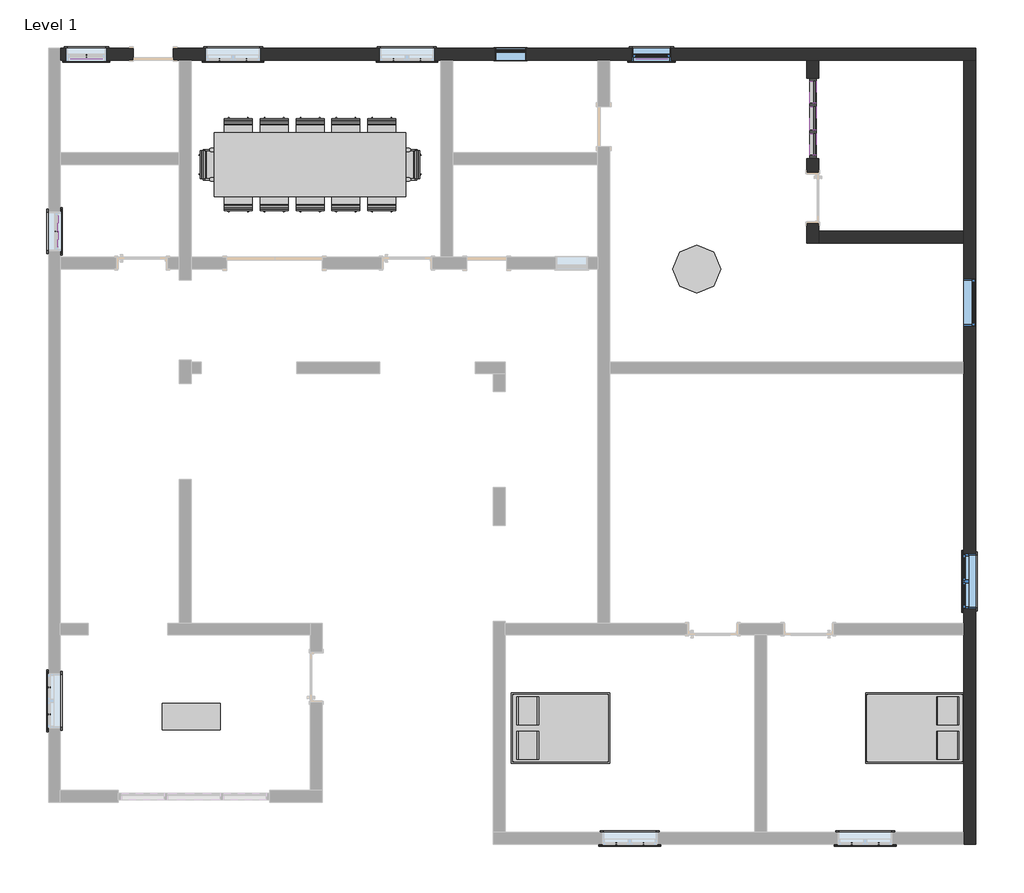
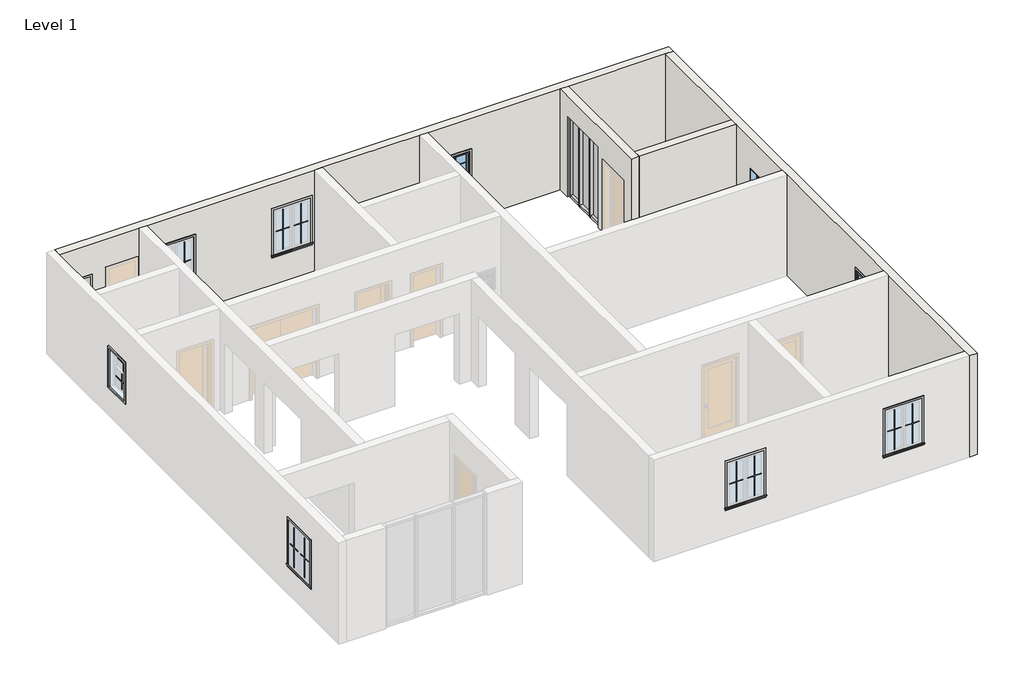
# One storey, part 2 of 2: 36 proxies, 17 furniture elements, 10 members, 4 walls, 4 windows, 3 plates.
"""IFC4 building model written with IfcOpenShell, lengths in millimetres."""

from ifc_helpers import new_model, si_unit, origin, origin_with_axes, place, context, project, spatial, polyline, outline, extrude, faceted_brep, transform, mapped, element, save
from components import muntin_pattern_2x2_muntin_pattern_2x2_88bf7f41, muntin_pattern_2x2_muntin_pattern_2x2_3dfd0a47, muntin_pattern_2x2_muntin_pattern_2x2_b8ba09c9, trim_window_exterior_flat_with_sill_4930676f, trim_window_exterior_flat_with_sill_6cd3ad68, trim_window_interior_flat_picture_frame_dd064338, trim_window_interior_flat_picture_frame_840a62db, furniture_b58f7881, chair_task_chair_task_b7f3823b, chair_task_arms_chair_task_arms_fa5a08ef, furniture_74675f9f, furniture_00fa8475, furniture_52f35bf4, member_05170f4c, member_f0fea5a5, member_24b1c93a, member_ee409385, system_panel_glazed_1f7552f7, system_panel_glazed_383feac9, window_c1f32544, window_c95ebb39, window_d400040f, window_f2d8fef0

model = new_model("IFC4")

# Units and contexts
model_context = context("Model", 3, world=origin())
ifc_project = project(units=[si_unit("LENGTHUNIT", "METRE", prefix="MILLI")], contexts=[model_context])

# Site, building, storey
site = spatial("IfcSite", under=ifc_project)
building = spatial("IfcBuilding", under=site)
storey = spatial("IfcBuildingStorey", under=building, Name="Level 1", Elevation=0.0)

# Proxies
placement = place(None, origin())
muntin_pattern_2x2_muntin_pattern_2x2_shape = muntin_pattern_2x2_muntin_pattern_2x2_88bf7f41(model_context)
element("IfcBuildingElementProxy", 1, Name="Muntin Pattern_2x2 : Muntin Pattern_2x2", ObjectType="Muntin Pattern_2x2 : Muntin Pattern_2x2", at=placement, inside=storey, context=model_context, shape_type="MappedRepresentation", body=[
    mapped(muntin_pattern_2x2_muntin_pattern_2x2_shape, transform((-3681.6839291, -4572.3847851, 984.25), x_axis=(-1.0, 0.0, 0.0), y_axis=(0.0, -1.0, 0.0), z_axis=(0.0, 0.0, 1.0))),
])
element("IfcBuildingElementProxy", 2, Name="Muntin Pattern_2x2 : Muntin Pattern_2x2", ObjectType="Muntin Pattern_2x2 : Muntin Pattern_2x2", at=placement, inside=storey, context=model_context, shape_type="MappedRepresentation", body=[
    mapped(muntin_pattern_2x2_muntin_pattern_2x2_shape, transform((818.2832584, -4572.3847851, 984.25), x_axis=(-1.0, 0.0, 0.0), y_axis=(0.0, -1.0, 0.0), z_axis=(0.0, 0.0, 1.0))),
])
element("IfcBuildingElementProxy", 3, Name="Muntin Pattern_2x2 : Muntin Pattern_2x2", ObjectType="Muntin Pattern_2x2 : Muntin Pattern_2x2", at=placement, inside=storey, context=model_context, shape_type="MappedRepresentation", body=[
    mapped(muntin_pattern_2x2_muntin_pattern_2x2_shape, transform((2454.7477116, 188.0316212, 984.25), x_axis=(0.0, 1.0, 0.0), y_axis=(-1.0, 0.0, 0.0), z_axis=(0.0, 0.0, 1.0))),
])
element("IfcBuildingElementProxy", 4, Name="Muntin Pattern_2x2 : Muntin Pattern_2x2", ObjectType="Muntin Pattern_2x2 : Muntin Pattern_2x2", at=placement, inside=storey, context=model_context, shape_type="MappedRepresentation", body=[
    mapped(muntin_pattern_2x2_muntin_pattern_2x2_shape, transform((-15045.2569759, -2097.9683788, 984.25), x_axis=(0.0, 1.0, 0.0), y_axis=(-1.0, 0.0, 0.0), z_axis=(0.0, 0.0, 1.0))),
])
element("IfcBuildingElementProxy", 5, Name="Muntin Pattern_2x2 : Muntin Pattern_2x2", ObjectType="Muntin Pattern_2x2 : Muntin Pattern_2x2", at=placement, inside=storey, context=model_context, shape_type="MappedRepresentation", body=[
    mapped(muntin_pattern_2x2_muntin_pattern_2x2_shape, transform((-11267.3046322, 10427.7042774, 984.25), x_axis=(-1.0, 0.0, 0.0), y_axis=(0.0, -1.0, 0.0), z_axis=(0.0, 0.0, 1.0))),
])
element("IfcBuildingElementProxy", 6, Name="Muntin Pattern_2x2 : Muntin Pattern_2x2", ObjectType="Muntin Pattern_2x2 : Muntin Pattern_2x2", at=placement, inside=storey, context=model_context, shape_type="MappedRepresentation", body=[
    mapped(muntin_pattern_2x2_muntin_pattern_2x2_shape, transform((-7943.6749447, 10427.7042774, 984.25), x_axis=(-1.0, 0.0, 0.0), y_axis=(0.0, -1.0, 0.0), z_axis=(0.0, 0.0, 1.0))),
])
muntin_pattern_2x2_muntin_pattern_2x2_2_shape = muntin_pattern_2x2_muntin_pattern_2x2_3dfd0a47(model_context)
element("IfcBuildingElementProxy", 7, Name="Muntin Pattern_2x2 : Muntin Pattern_2x2", ObjectType="Muntin Pattern_2x2 : Muntin Pattern_2x2", at=placement, inside=storey, context=model_context, shape_type="MappedRepresentation", body=[
    mapped(muntin_pattern_2x2_muntin_pattern_2x2_2_shape, transform((-4199.2089291, -4572.3847851, 984.25), x_axis=(1.0, 0.0, 0.0), y_axis=(0.0, 1.0, 0.0), z_axis=(0.0, 0.0, 1.0))),
])
element("IfcBuildingElementProxy", 8, Name="Muntin Pattern_2x2 : Muntin Pattern_2x2", ObjectType="Muntin Pattern_2x2 : Muntin Pattern_2x2", at=placement, inside=storey, context=model_context, shape_type="MappedRepresentation", body=[
    mapped(muntin_pattern_2x2_muntin_pattern_2x2_2_shape, transform((300.7582584, -4572.3847851, 984.25), x_axis=(1.0, 0.0, 0.0), y_axis=(0.0, 1.0, 0.0), z_axis=(0.0, 0.0, 1.0))),
])
element("IfcBuildingElementProxy", 9, Name="Muntin Pattern_2x2 : Muntin Pattern_2x2", ObjectType="Muntin Pattern_2x2 : Muntin Pattern_2x2", at=placement, inside=storey, context=model_context, shape_type="MappedRepresentation", body=[
    mapped(muntin_pattern_2x2_muntin_pattern_2x2_2_shape, transform((2454.7477116, 705.5566212, 984.25), x_axis=(0.0, -1.0, 0.0), y_axis=(1.0, 0.0, 0.0), z_axis=(0.0, 0.0, 1.0))),
])
element("IfcBuildingElementProxy", 10, Name="Muntin Pattern_2x2 : Muntin Pattern_2x2", ObjectType="Muntin Pattern_2x2 : Muntin Pattern_2x2", at=placement, inside=storey, context=model_context, shape_type="MappedRepresentation", body=[
    mapped(muntin_pattern_2x2_muntin_pattern_2x2_2_shape, transform((-15045.2569759, -1580.4433788, 984.25), x_axis=(0.0, -1.0, 0.0), y_axis=(1.0, 0.0, 0.0), z_axis=(0.0, 0.0, 1.0))),
])
element("IfcBuildingElementProxy", 11, Name="Muntin Pattern_2x2 : Muntin Pattern_2x2", ObjectType="Muntin Pattern_2x2 : Muntin Pattern_2x2", at=placement, inside=storey, context=model_context, shape_type="MappedRepresentation", body=[
    mapped(muntin_pattern_2x2_muntin_pattern_2x2_2_shape, transform((-11784.8296322, 10427.7042774, 984.25), x_axis=(1.0, 0.0, 0.0), y_axis=(0.0, 1.0, 0.0), z_axis=(0.0, 0.0, 1.0))),
])
element("IfcBuildingElementProxy", 12, Name="Muntin Pattern_2x2 : Muntin Pattern_2x2", ObjectType="Muntin Pattern_2x2 : Muntin Pattern_2x2", at=placement, inside=storey, context=model_context, shape_type="MappedRepresentation", body=[
    mapped(muntin_pattern_2x2_muntin_pattern_2x2_2_shape, transform((-8461.1999447, 10427.7042774, 984.25), x_axis=(1.0, 0.0, 0.0), y_axis=(0.0, 1.0, 0.0), z_axis=(0.0, 0.0, 1.0))),
])
muntin_pattern_2x2_muntin_pattern_2x2_3_shape = muntin_pattern_2x2_muntin_pattern_2x2_b8ba09c9(model_context)
element("IfcBuildingElementProxy", 13, Name="Muntin Pattern_2x2 : Muntin Pattern_2x2", ObjectType="Muntin Pattern_2x2 : Muntin Pattern_2x2", at=placement, inside=storey, context=model_context, shape_type="MappedRepresentation", body=[
    mapped(muntin_pattern_2x2_muntin_pattern_2x2_3_shape, transform((-14861.1069759, 7141.9761524, 1520.825), x_axis=(0.0, -1.0, 0.0), y_axis=(1.0, 0.0, 0.0), z_axis=(0.0, 0.0, 1.0))),
])
element("IfcBuildingElementProxy", 14, Name="Muntin Pattern_2x2 : Muntin Pattern_2x2", ObjectType="Muntin Pattern_2x2 : Muntin Pattern_2x2", at=placement, inside=storey, context=model_context, shape_type="MappedRepresentation", body=[
    mapped(muntin_pattern_2x2_muntin_pattern_2x2_3_shape, transform((-14905.5569759, 7141.9761524, 990.6), x_axis=(0.0, -1.0, 0.0), y_axis=(1.0, 0.0, 0.0), z_axis=(0.0, 0.0, 1.0))),
])
element("IfcBuildingElementProxy", 15, Name="Muntin Pattern_2x2 : Muntin Pattern_2x2", ObjectType="Muntin Pattern_2x2 : Muntin Pattern_2x2", at=placement, inside=storey, context=model_context, shape_type="MappedRepresentation", body=[
    mapped(muntin_pattern_2x2_muntin_pattern_2x2_3_shape, transform((-14330.8819759, 10453.1042774, 1520.825), x_axis=(-1.0, 0.0, 0.0), y_axis=(0.0, -1.0, 0.0), z_axis=(0.0, 0.0, 1.0))),
])
element("IfcBuildingElementProxy", 16, Name="Muntin Pattern_2x2 : Muntin Pattern_2x2", ObjectType="Muntin Pattern_2x2 : Muntin Pattern_2x2", at=placement, inside=storey, context=model_context, shape_type="MappedRepresentation", body=[
    mapped(muntin_pattern_2x2_muntin_pattern_2x2_3_shape, transform((-14330.8819759, 10497.5542774, 990.6), x_axis=(-1.0, 0.0, 0.0), y_axis=(0.0, -1.0, 0.0), z_axis=(0.0, 0.0, 1.0))),
])
element("IfcBuildingElementProxy", 17, Name="Muntin Pattern_2x2 : Muntin Pattern_2x2", ObjectType="Muntin Pattern_2x2 : Muntin Pattern_2x2", at=placement, inside=storey, context=model_context, shape_type="MappedRepresentation", body=[
    mapped(muntin_pattern_2x2_muntin_pattern_2x2_3_shape, transform((-3526.0593197, 10453.1042774, 1520.825), x_axis=(-1.0, 0.0, 0.0), y_axis=(0.0, -1.0, 0.0), z_axis=(0.0, 0.0, 1.0))),
])
element("IfcBuildingElementProxy", 18, Name="Muntin Pattern_2x2 : Muntin Pattern_2x2", ObjectType="Muntin Pattern_2x2 : Muntin Pattern_2x2", at=placement, inside=storey, context=model_context, shape_type="MappedRepresentation", body=[
    mapped(muntin_pattern_2x2_muntin_pattern_2x2_3_shape, transform((-3526.0593197, 10497.5542774, 990.6), x_axis=(-1.0, 0.0, 0.0), y_axis=(0.0, -1.0, 0.0), z_axis=(0.0, 0.0, 1.0))),
])
trim_window_exterior_flat_with_sill_shape = trim_window_exterior_flat_with_sill_4930676f(model_context)
element("IfcBuildingElementProxy", 19, Name="Trim-Window-Exterior-Flat : with Sill", ObjectType="Trim-Window-Exterior-Flat : with Sill", at=placement, inside=storey, context=model_context, shape_type="MappedRepresentation", body=[
    mapped(trim_window_exterior_flat_with_sill_shape, transform((-3940.4464291, -4581.9097851, 2260.6), x_axis=(1.0, 0.0, 0.0), y_axis=(0.0, 0.0, 1.0), z_axis=(0.0, -1.0, 0.0))),
])
element("IfcBuildingElementProxy", 20, Name="Trim-Window-Exterior-Flat : with Sill", ObjectType="Trim-Window-Exterior-Flat : with Sill", at=placement, inside=storey, context=model_context, shape_type="MappedRepresentation", body=[
    mapped(trim_window_exterior_flat_with_sill_shape, transform((559.5207584, -4581.9097851, 2260.6), x_axis=(1.0, 0.0, 0.0), y_axis=(0.0, 0.0, 1.0), z_axis=(0.0, -1.0, 0.0))),
])
element("IfcBuildingElementProxy", 21, Name="Trim-Window-Exterior-Flat : with Sill", ObjectType="Trim-Window-Exterior-Flat : with Sill", at=placement, inside=storey, context=model_context, shape_type="MappedRepresentation", body=[
    mapped(trim_window_exterior_flat_with_sill_shape, transform((2445.2227116, 446.7941212, 2260.6), x_axis=(0.0, -1.0, 0.0), y_axis=(0.0, 0.0, 1.0), z_axis=(-1.0, 0.0, 0.0))),
])
element("IfcBuildingElementProxy", 22, Name="Trim-Window-Exterior-Flat : with Sill", ObjectType="Trim-Window-Exterior-Flat : with Sill", at=placement, inside=storey, context=model_context, shape_type="MappedRepresentation", body=[
    mapped(trim_window_exterior_flat_with_sill_shape, transform((-15054.7819759, -1839.2058788, 2260.6), x_axis=(0.0, -1.0, 0.0), y_axis=(0.0, 0.0, 1.0), z_axis=(-1.0, 0.0, 0.0))),
])
element("IfcBuildingElementProxy", 23, Name="Trim-Window-Exterior-Flat : with Sill", ObjectType="Trim-Window-Exterior-Flat : with Sill", at=placement, inside=storey, context=model_context, shape_type="MappedRepresentation", body=[
    mapped(trim_window_exterior_flat_with_sill_shape, transform((-11526.0671322, 10418.1792774, 2260.6), x_axis=(1.0, 0.0, 0.0), y_axis=(0.0, 0.0, 1.0), z_axis=(0.0, -1.0, 0.0))),
])
element("IfcBuildingElementProxy", 24, Name="Trim-Window-Exterior-Flat : with Sill", ObjectType="Trim-Window-Exterior-Flat : with Sill", at=placement, inside=storey, context=model_context, shape_type="MappedRepresentation", body=[
    mapped(trim_window_exterior_flat_with_sill_shape, transform((-8202.4374447, 10418.1792774, 2260.6), x_axis=(1.0, 0.0, 0.0), y_axis=(0.0, 0.0, 1.0), z_axis=(0.0, -1.0, 0.0))),
])
trim_window_exterior_flat_with_sill_2_shape = trim_window_exterior_flat_with_sill_6cd3ad68(model_context)
element("IfcBuildingElementProxy", 25, Name="Trim-Window-Exterior-Flat : with Sill", ObjectType="Trim-Window-Exterior-Flat : with Sill", at=placement, inside=storey, context=model_context, shape_type="MappedRepresentation", body=[
    mapped(trim_window_exterior_flat_with_sill_2_shape, transform((-14826.1819759, 7141.9761524, 2082.8), x_axis=(0.0, 1.0, 0.0), y_axis=(0.0, 0.0, 1.0), z_axis=(1.0, 0.0, 0.0))),
])
element("IfcBuildingElementProxy", 26, Name="Trim-Window-Exterior-Flat : with Sill", ObjectType="Trim-Window-Exterior-Flat : with Sill", at=placement, inside=storey, context=model_context, shape_type="MappedRepresentation", body=[
    mapped(trim_window_exterior_flat_with_sill_2_shape, transform((-14330.8819759, 10418.1792774, 2082.8), x_axis=(1.0, 0.0, 0.0), y_axis=(0.0, 0.0, 1.0), z_axis=(0.0, -1.0, 0.0))),
])
element("IfcBuildingElementProxy", 27, Name="Trim-Window-Exterior-Flat : with Sill", ObjectType="Trim-Window-Exterior-Flat : with Sill", at=placement, inside=storey, context=model_context, shape_type="MappedRepresentation", body=[
    mapped(trim_window_exterior_flat_with_sill_2_shape, transform((-3526.0593197, 10418.1792774, 2082.8), x_axis=(1.0, 0.0, 0.0), y_axis=(0.0, 0.0, 1.0), z_axis=(0.0, -1.0, 0.0))),
])
trim_window_interior_flat_picture_frame_shape = trim_window_interior_flat_picture_frame_dd064338(model_context)
element("IfcBuildingElementProxy", 28, Name="Trim-Window-Interior-Flat : Picture Frame", ObjectType="Trim-Window-Interior-Flat : Picture Frame", at=placement, inside=storey, context=model_context, shape_type="MappedRepresentation", body=[
    mapped(trim_window_interior_flat_picture_frame_shape, transform((-3940.4464291, -4353.3097851, 2260.6), x_axis=(-1.0, 0.0, 0.0), y_axis=(0.0, 0.0, 1.0), z_axis=(0.0, 1.0, 0.0))),
])
element("IfcBuildingElementProxy", 29, Name="Trim-Window-Interior-Flat : Picture Frame", ObjectType="Trim-Window-Interior-Flat : Picture Frame", at=placement, inside=storey, context=model_context, shape_type="MappedRepresentation", body=[
    mapped(trim_window_interior_flat_picture_frame_shape, transform((559.5207584, -4353.3097851, 2260.6), x_axis=(-1.0, 0.0, 0.0), y_axis=(0.0, 0.0, 1.0), z_axis=(0.0, 1.0, 0.0))),
])
element("IfcBuildingElementProxy", 30, Name="Trim-Window-Interior-Flat : Picture Frame", ObjectType="Trim-Window-Interior-Flat : Picture Frame", at=placement, inside=storey, context=model_context, shape_type="MappedRepresentation", body=[
    mapped(trim_window_interior_flat_picture_frame_shape, transform((2673.8227116, 446.7941212, 2260.6), x_axis=(0.0, 1.0, 0.0), y_axis=(0.0, 0.0, 1.0), z_axis=(1.0, 0.0, 0.0))),
])
element("IfcBuildingElementProxy", 31, Name="Trim-Window-Interior-Flat : Picture Frame", ObjectType="Trim-Window-Interior-Flat : Picture Frame", at=placement, inside=storey, context=model_context, shape_type="MappedRepresentation", body=[
    mapped(trim_window_interior_flat_picture_frame_shape, transform((-14826.1819759, -1839.2058788, 2260.6), x_axis=(0.0, 1.0, 0.0), y_axis=(0.0, 0.0, 1.0), z_axis=(1.0, 0.0, 0.0))),
])
element("IfcBuildingElementProxy", 32, Name="Trim-Window-Interior-Flat : Picture Frame", ObjectType="Trim-Window-Interior-Flat : Picture Frame", at=placement, inside=storey, context=model_context, shape_type="MappedRepresentation", body=[
    mapped(trim_window_interior_flat_picture_frame_shape, transform((-11526.0671322, 10646.7792774, 2260.6), x_axis=(-1.0, 0.0, 0.0), y_axis=(0.0, 0.0, 1.0), z_axis=(0.0, 1.0, 0.0))),
])
element("IfcBuildingElementProxy", 33, Name="Trim-Window-Interior-Flat : Picture Frame", ObjectType="Trim-Window-Interior-Flat : Picture Frame", at=placement, inside=storey, context=model_context, shape_type="MappedRepresentation", body=[
    mapped(trim_window_interior_flat_picture_frame_shape, transform((-8202.4374447, 10646.7792774, 2260.6), x_axis=(-1.0, 0.0, 0.0), y_axis=(0.0, 0.0, 1.0), z_axis=(0.0, 1.0, 0.0))),
])
trim_window_interior_flat_picture_frame_2_shape = trim_window_interior_flat_picture_frame_840a62db(model_context)
element("IfcBuildingElementProxy", 34, Name="Trim-Window-Interior-Flat : Picture Frame", ObjectType="Trim-Window-Interior-Flat : Picture Frame", at=placement, inside=storey, context=model_context, shape_type="MappedRepresentation", body=[
    mapped(trim_window_interior_flat_picture_frame_2_shape, transform((-15054.7819759, 7141.9761524, 2082.8), x_axis=(0.0, -1.0, 0.0), y_axis=(0.0, 0.0, 1.0), z_axis=(-1.0, 0.0, 0.0))),
])
element("IfcBuildingElementProxy", 35, Name="Trim-Window-Interior-Flat : Picture Frame", ObjectType="Trim-Window-Interior-Flat : Picture Frame", at=placement, inside=storey, context=model_context, shape_type="MappedRepresentation", body=[
    mapped(trim_window_interior_flat_picture_frame_2_shape, transform((-14330.8819759, 10646.7792774, 2082.8), x_axis=(-1.0, 0.0, 0.0), y_axis=(0.0, 0.0, 1.0), z_axis=(0.0, 1.0, 0.0))),
])
element("IfcBuildingElementProxy", 36, Name="Trim-Window-Interior-Flat : Picture Frame", ObjectType="Trim-Window-Interior-Flat : Picture Frame", at=placement, inside=storey, context=model_context, shape_type="MappedRepresentation", body=[
    mapped(trim_window_interior_flat_picture_frame_2_shape, transform((-3526.0593197, 10646.7792774, 2082.8), x_axis=(-1.0, 0.0, 0.0), y_axis=(0.0, 0.0, 1.0), z_axis=(0.0, 1.0, 0.0))),
])

# Furniture
furniture_shape = furniture_b58f7881(model_context)
element("IfcFurniture", 37, ObjectType="Bed-Box : Double 53\" x 74\"", at=placement, inside=storey, context=model_context, shape_type="MappedRepresentation", body=[
    mapped(furniture_shape, transform((-5500.3888279, -2699.0583378, 0.0), x_axis=(0.0, 1.0, 0.0), y_axis=(-1.0, 0.0, 0.0), z_axis=(0.0, 0.0, 1.0))),
])
element("IfcFurniture", 38, ObjectType="Bed-Box : Double 53\" x 74\"", at=placement, inside=storey, context=model_context, shape_type="MappedRepresentation", body=[
    mapped(furniture_shape, transform((1739.8522198, -2020.7534198, 0.0), x_axis=(0.0, -1.0, 0.0), y_axis=(1.0, 0.0, 0.0), z_axis=(0.0, 0.0, 1.0))),
])
chair_task_chair_task_shape = chair_task_chair_task_b7f3823b(model_context)
element("IfcFurniture", 39, ObjectType="Chair-Task : Chair-Task", at=placement, inside=storey, context=model_context, shape_type="MappedRepresentation", body=[
    mapped(chair_task_chair_task_shape, transform((-9227.9614688, 9046.5743978, 0.0), x_axis=(-1.0, 0.0, 0.0), y_axis=(0.0, -1.0, 0.0), z_axis=(0.0, 0.0, 1.0))),
])
element("IfcFurniture", 40, ObjectType="Chair-Task : Chair-Task", at=placement, inside=storey, context=model_context, shape_type="MappedRepresentation", body=[
    mapped(chair_task_chair_task_shape, transform((-9509.9431081, 7789.4825945, 0.0), x_axis=(1.0, 0.0, 0.0), y_axis=(0.0, 1.0, 0.0), z_axis=(0.0, 0.0, 1.0))),
])
element("IfcFurniture", 41, ObjectType="Chair-Task : Chair-Task", at=placement, inside=storey, context=model_context, shape_type="MappedRepresentation", body=[
    mapped(chair_task_chair_task_shape, transform((-9913.7614688, 9046.5743978, 0.0), x_axis=(-1.0, 0.0, 0.0), y_axis=(0.0, -1.0, 0.0), z_axis=(0.0, 0.0, 1.0))),
])
element("IfcFurniture", 42, ObjectType="Chair-Task : Chair-Task", at=placement, inside=storey, context=model_context, shape_type="MappedRepresentation", body=[
    mapped(chair_task_chair_task_shape, transform((-10195.7431081, 7789.4825945, 0.0), x_axis=(1.0, 0.0, 0.0), y_axis=(0.0, 1.0, 0.0), z_axis=(0.0, 0.0, 1.0))),
])
element("IfcFurniture", 43, ObjectType="Chair-Task : Chair-Task", at=placement, inside=storey, context=model_context, shape_type="MappedRepresentation", body=[
    mapped(chair_task_chair_task_shape, transform((-10599.5614688, 9046.5743978, 0.0), x_axis=(-1.0, 0.0, 0.0), y_axis=(0.0, -1.0, 0.0), z_axis=(0.0, 0.0, 1.0))),
])
element("IfcFurniture", 44, ObjectType="Chair-Task : Chair-Task", at=placement, inside=storey, context=model_context, shape_type="MappedRepresentation", body=[
    mapped(chair_task_chair_task_shape, transform((-8542.1614688, 9046.5743978, 0.0), x_axis=(-1.0, 0.0, 0.0), y_axis=(0.0, -1.0, 0.0), z_axis=(0.0, 0.0, 1.0))),
])
element("IfcFurniture", 45, ObjectType="Chair-Task : Chair-Task", at=placement, inside=storey, context=model_context, shape_type="MappedRepresentation", body=[
    mapped(chair_task_chair_task_shape, transform((-10881.5431081, 7789.4825945, 0.0), x_axis=(1.0, 0.0, 0.0), y_axis=(0.0, 1.0, 0.0), z_axis=(0.0, 0.0, 1.0))),
])
element("IfcFurniture", 46, ObjectType="Chair-Task : Chair-Task", at=placement, inside=storey, context=model_context, shape_type="MappedRepresentation", body=[
    mapped(chair_task_chair_task_shape, transform((-8824.1431081, 7789.4825945, 0.0), x_axis=(1.0, 0.0, 0.0), y_axis=(0.0, 1.0, 0.0), z_axis=(0.0, 0.0, 1.0))),
])
element("IfcFurniture", 47, ObjectType="Chair-Task : Chair-Task", at=placement, inside=storey, context=model_context, shape_type="MappedRepresentation", body=[
    mapped(chair_task_chair_task_shape, transform((-11285.3614688, 9046.5743978, 0.0), x_axis=(-1.0, 0.0, 0.0), y_axis=(0.0, -1.0, 0.0), z_axis=(0.0, 0.0, 1.0))),
])
element("IfcFurniture", 48, ObjectType="Chair-Task : Chair-Task", at=placement, inside=storey, context=model_context, shape_type="MappedRepresentation", body=[
    mapped(chair_task_chair_task_shape, transform((-11567.3431081, 7789.4825945, 0.0), x_axis=(1.0, 0.0, 0.0), y_axis=(0.0, 1.0, 0.0), z_axis=(0.0, 0.0, 1.0))),
])
chair_task_arms_chair_task_arms_shape = chair_task_arms_chair_task_arms_fa5a08ef(model_context)
element("IfcFurniture", 49, ObjectType="Chair-Task Arms : Chair-Task Arms", at=placement, inside=storey, context=model_context, shape_type="MappedRepresentation", body=[
    mapped(chair_task_arms_chair_task_arms_shape, transform((-11902.4981901, 8559.0193159, 0.0), x_axis=(0.0, -1.0, 0.0), y_axis=(1.0, 0.0, 0.0), z_axis=(0.0, 0.0, 1.0))),
])
element("IfcFurniture", 50, ObjectType="Chair-Task Arms : Chair-Task Arms", at=placement, inside=storey, context=model_context, shape_type="MappedRepresentation", body=[
    mapped(chair_task_arms_chair_task_arms_shape, transform((-8207.0063868, 8277.0376765, 0.0), x_axis=(0.0, 1.0, 0.0), y_axis=(-1.0, 0.0, 0.0), z_axis=(0.0, 0.0, 1.0))),
])
furniture_2_shape = furniture_74675f9f(model_context)
element("IfcFurniture", 51, ObjectType="Table-Coffee Mission : 44\" x 20\"", at=placement, inside=storey, context=model_context, shape_type="MappedRepresentation", body=[
    mapped(furniture_2_shape, transform((-12326.1671322, -2144.0058788, 0.0), x_axis=(1.0, 0.0, 0.0), y_axis=(0.0, 1.0, 0.0), z_axis=(0.0, 0.0, 1.0))),
])
furniture_3_shape = furniture_00fa8475(model_context)
element("IfcFurniture", 52, ObjectType="Table-Conference2 w Chairs : 48\" x 144\"", at=placement, inside=storey, context=model_context, shape_type="MappedRepresentation", body=[
    mapped(furniture_3_shape, transform((-10054.7522884, 8418.0284962, 0.0), x_axis=(1.0, 0.0, 0.0), y_axis=(0.0, 1.0, 0.0), z_axis=(0.0, 0.0, 1.0))),
])
furniture_4_shape = furniture_52f35bf4(model_context)
element("IfcFurniture", 53, ObjectType="Table-Dining Round w Chairs : 36\" Diameter", at=placement, inside=storey, context=model_context, shape_type="MappedRepresentation", body=[
    mapped(furniture_4_shape, transform((-2763.3631619, 6602.954841, 0.0), x_axis=(1.0, 0.0, 0.0), y_axis=(0.0, 1.0, 0.0), z_axis=(0.0, 0.0, 1.0))),
])

# Members
member_shape = member_05170f4c(model_context)
element("IfcMember", 54, ObjectType="Rectangular Mullion : 2.5\" x 5\" rectangular", at=placement, inside=storey, context=model_context, shape_type="MappedRepresentation", body=[
    mapped(member_shape, transform((-440.4554134, 8595.8284962, 2438.4), x_axis=(0.0, 0.0, 1.0), y_axis=(-1.0, 0.0, 0.0), z_axis=(0.0, -1.0, 0.0))),
])
element("IfcMember", 55, ObjectType="Rectangular Mullion : 2.5\" x 5\" rectangular", at=placement, inside=storey, context=model_context, shape_type="MappedRepresentation", body=[
    mapped(member_shape, transform((-440.4554134, 9592.7123504, 2438.4), x_axis=(0.0, 0.0, 1.0), y_axis=(-1.0, 0.0, 0.0), z_axis=(0.0, -1.0, 0.0))),
])
element("IfcMember", 56, ObjectType="Rectangular Mullion : 2.5\" x 5\" rectangular", at=placement, inside=storey, context=model_context, shape_type="MappedRepresentation", body=[
    mapped(member_shape, transform((-440.4554134, 10011.7792774, 0.0), x_axis=(0.0, 0.0, -1.0), y_axis=(-1.0, 0.0, 0.0), z_axis=(0.0, 1.0, 0.0))),
])
element("IfcMember", 57, ObjectType="Rectangular Mullion : 2.5\" x 5\" rectangular", at=placement, inside=storey, context=model_context, shape_type="MappedRepresentation", body=[
    mapped(member_shape, transform((-440.4554134, 9014.8954233, 0.0), x_axis=(0.0, 0.0, -1.0), y_axis=(-1.0, 0.0, 0.0), z_axis=(0.0, 1.0, 0.0))),
])
member_2_shape = member_f0fea5a5(model_context)
element("IfcMember", 58, ObjectType="Rectangular Mullion : 2.5\" x 5\" rectangular", at=placement, inside=storey, context=model_context, shape_type="MappedRepresentation", body=[
    mapped(member_2_shape, transform((-440.4554134, 9560.9623504, 0.0), x_axis=(0.0, -1.0, 0.0), y_axis=(-1.0, 0.0, 0.0), z_axis=(0.0, 0.0, -1.0))),
])
element("IfcMember", 59, ObjectType="Rectangular Mullion : 2.5\" x 5\" rectangular", at=placement, inside=storey, context=model_context, shape_type="MappedRepresentation", body=[
    mapped(member_2_shape, transform((-440.4554134, 9046.6454233, 0.0), x_axis=(0.0, -1.0, 0.0), y_axis=(-1.0, 0.0, 0.0), z_axis=(0.0, 0.0, -1.0))),
])
member_3_shape = member_24b1c93a(model_context)
element("IfcMember", 60, ObjectType="Rectangular Mullion : 2.5\" x 5\" rectangular", at=placement, inside=storey, context=model_context, shape_type="MappedRepresentation", body=[
    mapped(member_3_shape, transform((-440.4554134, 9529.2123504, 0.0), x_axis=(0.0, 0.0, -1.0), y_axis=(-1.0, 0.0, 0.0), z_axis=(0.0, 1.0, 0.0))),
])
element("IfcMember", 61, ObjectType="Rectangular Mullion : 2.5\" x 5\" rectangular", at=placement, inside=storey, context=model_context, shape_type="MappedRepresentation", body=[
    mapped(member_3_shape, transform((-440.4554134, 9078.3954233, 2438.4), x_axis=(0.0, 0.0, 1.0), y_axis=(-1.0, 0.0, 0.0), z_axis=(0.0, -1.0, 0.0))),
])
member_4_shape = member_ee409385(model_context)
element("IfcMember", 62, ObjectType="Rectangular Mullion : 2.5\" x 5\" rectangular", at=placement, inside=storey, context=model_context, shape_type="MappedRepresentation", body=[
    mapped(member_4_shape, transform((-440.4554134, 10075.2792774, 2438.4), x_axis=(0.0, 1.0, 0.0), y_axis=(-1.0, 0.0, 0.0), z_axis=(0.0, 0.0, 1.0))),
])
element("IfcMember", 63, ObjectType="Rectangular Mullion : 2.5\" x 5\" rectangular", at=placement, inside=storey, context=model_context, shape_type="MappedRepresentation", body=[
    mapped(member_4_shape, transform((-440.4554134, 8532.3284962, 0.0), x_axis=(0.0, -1.0, 0.0), y_axis=(-1.0, 0.0, 0.0), z_axis=(0.0, 0.0, -1.0))),
])

# Plates
system_panel_glazed_shape = system_panel_glazed_1f7552f7(model_context)
element("IfcPlate", 64, ObjectType="System Panel : Glazed", at=placement, inside=storey, context=model_context, shape_type="MappedRepresentation", body=[
    mapped(system_panel_glazed_shape, transform((-440.4554134, 9802.2458139, 63.5), x_axis=(0.0, -1.0, 0.0), y_axis=(1.0, 0.0, 0.0), z_axis=(0.0, 0.0, 1.0))),
])
element("IfcPlate", 65, ObjectType="System Panel : Glazed", at=placement, inside=storey, context=model_context, shape_type="MappedRepresentation", body=[
    mapped(system_panel_glazed_shape, transform((-440.4554134, 8805.3619597, 63.5), x_axis=(0.0, -1.0, 0.0), y_axis=(1.0, 0.0, 0.0), z_axis=(0.0, 0.0, 1.0))),
])
system_panel_glazed_2_shape = system_panel_glazed_383feac9(model_context)
element("IfcPlate", 66, ObjectType="System Panel : Glazed", at=placement, inside=storey, context=model_context, shape_type="MappedRepresentation", body=[
    mapped(system_panel_glazed_2_shape, transform((-440.4554134, 9303.8038868, 63.5), x_axis=(0.0, -1.0, 0.0), y_axis=(1.0, 0.0, 0.0), z_axis=(0.0, 0.0, 1.0))),
])

# Walls
element("IfcWall", 67, ObjectType="9\" wall", at=placement, inside=storey, context=model_context, shape_type="Brep", body=[
    faceted_brep([(-12669.0671322, 10418.1792774, 2133.6), (-12669.0671322, 10418.1792774, 0.0), (-12554.7671322, 10418.1792774, 0.0), (-12326.1671322, 10418.1792774, 0.0), (-7554.7374447, 10418.1792774, 0.0), (-7326.1374447, 10418.1792774, 0.0), (-4554.7593197, 10418.1792774, 0.0), (-4326.1593197, 10418.1792774, 0.0), (-554.7554134, 10418.1792774, 0.0), (-326.1554134, 10418.1792774, 0.0), (2445.2227116, 10418.1792774, 0.0), (2673.8227116, 10418.1792774, 0.0), (2673.8227116, 10418.1792774, 3048.0), (2445.2227116, 10418.1792774, 3048.0), (-326.1554134, 10418.1792774, 3048.0), (-554.7554134, 10418.1792774, 3048.0), (-4326.1593197, 10418.1792774, 3048.0), (-4554.7593197, 10418.1792774, 3048.0), (-7326.1374447, 10418.1792774, 3048.0), (-7554.7374447, 10418.1792774, 3048.0), (-12326.1671322, 10418.1792774, 3048.0), (-12554.7671322, 10418.1792774, 3048.0), (-14826.1819759, 10418.1792774, 3048.0), (-14826.1819759, 10418.1792774, 0.0), (-13431.0671322, 10418.1792774, 0.0), (-13431.0671322, 10418.1792774, 2133.6), (-12046.7671322, 10418.1792774, 2260.6), (-11005.3671322, 10418.1792774, 2260.6), (-11005.3671322, 10418.1792774, 914.4), (-12046.7671322, 10418.1792774, 914.4), (-8723.1374447, 10418.1792774, 2260.6), (-7681.7374447, 10418.1792774, 2260.6), (-7681.7374447, 10418.1792774, 914.4), (-8723.1374447, 10418.1792774, 914.4), (-6526.0374447, 10418.1792774, 1524.0), (-5916.4374447, 10418.1792774, 1524.0), (-5916.4374447, 10418.1792774, 914.4), (-6526.0374447, 10418.1792774, 914.4), (-13949.8819759, 10418.1792774, 2082.8), (-13949.8819759, 10418.1792774, 914.4), (-14711.8819759, 10418.1792774, 914.4), (-14711.8819759, 10418.1792774, 2082.8), (-3145.0593197, 10418.1792774, 2082.8), (-3145.0593197, 10418.1792774, 914.4), (-3907.0593197, 10418.1792774, 914.4), (-3907.0593197, 10418.1792774, 2082.8), (2673.8227116, 10646.7792774, 0.0), (-12669.0671322, 10646.7792774, 0.0), (-12669.0671322, 10646.7792774, 2133.6), (-13431.0671322, 10646.7792774, 2133.6), (-13431.0671322, 10646.7792774, 0.0), (-14826.1819759, 10646.7792774, 0.0), (-14826.1819759, 10646.7792774, 3048.0), (2673.8227116, 10646.7792774, 3048.0), (-12046.7671322, 10646.7792774, 2260.6), (-12046.7671322, 10646.7792774, 914.4), (-11005.3671322, 10646.7792774, 914.4), (-11005.3671322, 10646.7792774, 2260.6), (-8723.1374447, 10646.7792774, 2260.6), (-8723.1374447, 10646.7792774, 914.4), (-7681.7374447, 10646.7792774, 914.4), (-7681.7374447, 10646.7792774, 2260.6), (-6526.0374447, 10646.7792774, 1524.0), (-6526.0374447, 10646.7792774, 914.4), (-5916.4374447, 10646.7792774, 914.4), (-5916.4374447, 10646.7792774, 1524.0), (-13949.8819759, 10646.7792774, 2082.8), (-14711.8819759, 10646.7792774, 2082.8), (-14711.8819759, 10646.7792774, 914.4), (-13949.8819759, 10646.7792774, 914.4), (-3145.0593197, 10646.7792774, 2082.8), (-3907.0593197, 10646.7792774, 2082.8), (-3907.0593197, 10646.7792774, 914.4), (-3145.0593197, 10646.7792774, 914.4)], [[[0, 1, 2, 3, 4, 5, 6, 7, 8, 9, 10, 11, 12, 13, 14, 15, 16, 17, 18, 19, 20, 21, 22, 23, 24, 25], [26, 27, 28, 29], [30, 31, 32, 33], [34, 35, 36, 37], [38, 39, 40, 41], [42, 43, 44, 45]], [[46, 47, 48, 49, 50, 51, 52, 53], [54, 55, 56, 57], [58, 59, 60, 61], [62, 63, 64, 65], [66, 67, 68, 69], [70, 71, 72, 73]], [[24, 23, 51, 50]], [[11, 10, 9, 8, 7, 6, 5, 4, 3, 2, 1, 47, 46]], [[22, 21, 20, 19, 18, 17, 16, 15, 14, 13, 12, 53, 52]], [[23, 22, 52, 51]], [[12, 11, 46, 53]], [[55, 54, 26, 29]], [[56, 55, 29, 28]], [[57, 56, 28, 27]], [[54, 57, 27, 26]], [[59, 58, 30, 33]], [[60, 59, 33, 32]], [[61, 60, 32, 31]], [[58, 61, 31, 30]], [[63, 62, 34, 37]], [[64, 63, 37, 36]], [[65, 64, 36, 35]], [[62, 65, 35, 34]], [[39, 38, 66, 69]], [[40, 39, 69, 68]], [[41, 40, 68, 67]], [[38, 41, 67, 66]], [[43, 42, 70, 73]], [[44, 43, 73, 72]], [[45, 44, 72, 71]], [[42, 45, 71, 70]], [[48, 47, 1, 0]], [[49, 48, 0, 25]], [[50, 49, 25, 24]]]),
])
element("IfcWall", 68, ObjectType="9\" wall", at=placement, inside=storey, context=model_context, shape_type="Brep", body=[
    faceted_brep([(2445.2227116, 10418.1792774, 0.0), (2445.2227116, 7146.7386524, 0.0), (2445.2227116, 6918.1386524, 0.0), (2445.2227116, 4646.7238087, 0.0), (2445.2227116, 4418.1238087, 0.0), (2445.2227116, -353.3058788, 0.0), (2445.2227116, -581.9058788, 0.0), (2445.2227116, -4353.3097851, 0.0), (2445.2227116, -4581.9097851, 0.0), (2445.2227116, -4581.9097851, 3048.0), (2445.2227116, -4353.3097851, 3048.0), (2445.2227116, -581.9058788, 3048.0), (2445.2227116, -353.3058788, 3048.0), (2445.2227116, 4418.1238087, 3048.0), (2445.2227116, 4646.7238087, 3048.0), (2445.2227116, 6918.1386524, 3048.0), (2445.2227116, 7146.7386524, 3048.0), (2445.2227116, 10418.1792774, 3048.0), (2445.2227116, 5325.2312306, 2133.6), (2445.2227116, 5325.2312306, 914.4), (2445.2227116, 6239.6312306, 914.4), (2445.2227116, 6239.6312306, 2133.6), (2445.2227116, 967.4941212, 2260.6), (2445.2227116, -73.9058788, 2260.6), (2445.2227116, -73.9058788, 914.4), (2445.2227116, 967.4941212, 914.4), (2673.8227116, 10418.1792774, 0.0), (2673.8227116, 10418.1792774, 3048.0), (2673.8227116, -4581.9097851, 3048.0), (2673.8227116, -4581.9097851, 0.0), (2673.8227116, 5325.2312306, 2133.6), (2673.8227116, 6239.6312306, 2133.6), (2673.8227116, 6239.6312306, 914.4), (2673.8227116, 5325.2312306, 914.4), (2673.8227116, 967.4941212, 2260.6), (2673.8227116, 967.4941212, 914.4), (2673.8227116, -73.9058788, 914.4), (2673.8227116, -73.9058788, 2260.6)], [[[0, 1, 2, 3, 4, 5, 6, 7, 8, 9, 10, 11, 12, 13, 14, 15, 16, 17], [18, 19, 20, 21], [22, 23, 24, 25]], [[26, 27, 28, 29], [30, 31, 32, 33], [34, 35, 36, 37]], [[8, 7, 6, 5, 4, 3, 2, 1, 0, 26, 29]], [[17, 16, 15, 14, 13, 12, 11, 10, 9, 28, 27]], [[0, 17, 27, 26]], [[9, 8, 29, 28]], [[19, 18, 30, 33]], [[20, 19, 33, 32]], [[21, 20, 32, 31]], [[18, 21, 31, 30]], [[35, 34, 22, 25]], [[36, 35, 25, 24]], [[37, 36, 24, 23]], [[34, 37, 23, 22]]]),
])
element("IfcWall", 69, ObjectType="9\" wall", at=placement, inside=storey, context=model_context, shape_type="Brep", body=[
    faceted_brep([(-554.7554134, 6918.1386524, 3048.0), (-554.7554134, 10418.1792774, 3048.0), (-554.7554134, 10418.1792774, 0.0), (-554.7554134, 10075.2792774, 0.0), (-554.7554134, 10075.2792774, 2438.4), (-554.7554134, 8532.3284962, 2438.4), (-554.7554134, 8532.3284962, 0.0), (-554.7554134, 8264.9835743, 0.0), (-554.7554134, 8264.9835743, 2159.0), (-554.7554134, 7299.7835743, 2159.0), (-554.7554134, 7299.7835743, 0.0), (-554.7554134, 6918.1386524, 0.0), (-326.1554134, 10418.1792774, 3048.0), (-326.1554134, 7146.7386524, 3048.0), (-326.1554134, 6918.1386524, 3048.0), (-326.1554134, 6918.1386524, 0.0), (-326.1554134, 7146.7386524, 0.0), (-326.1554134, 7299.7835743, 0.0), (-326.1554134, 7299.7835743, 2159.0), (-326.1554134, 8264.9835743, 2159.0), (-326.1554134, 8264.9835743, 0.0), (-326.1554134, 8532.3284962, 0.0), (-326.1554134, 8532.3284962, 2438.4), (-326.1554134, 10075.2792774, 2438.4), (-326.1554134, 10075.2792774, 0.0), (-326.1554134, 10418.1792774, 0.0)], [[[0, 1, 2, 3, 4, 5, 6, 7, 8, 9, 10, 11]], [[12, 13, 14, 15, 16, 17, 18, 19, 20, 21, 22, 23, 24, 25]], [[2, 25, 24, 3]], [[15, 11, 10, 17, 16]], [[20, 7, 6, 21]], [[1, 0, 14, 13, 12]], [[2, 1, 12, 25]], [[0, 11, 15, 14]], [[23, 4, 3, 24]], [[4, 23, 22, 5]], [[5, 22, 21, 6]], [[9, 18, 17, 10]], [[18, 9, 8, 19]], [[19, 8, 7, 20]]]),
])
element("IfcWall", 70, ObjectType="9\" wall", at=placement, inside=storey, context=model_context, shape_type="SweptSolid", body=[
    extrude(outline(polyline([(2445.2227116, 6918.1386524), (-326.1554134, 6918.1386524), (-326.1554134, 7146.7386524), (2445.2227116, 7146.7386524), (2445.2227116, 6918.1386524)])), origin_with_axes(), (0.0, 0.0, 1.0), 3048.0),
])

# Windows
window_shape = window_c1f32544(model_context)
element("IfcWindow", 71, ObjectType="Fixed : 36\" x 48\"", at=placement, inside=storey, context=model_context, shape_type="MappedRepresentation", body=[
    mapped(window_shape, transform((2559.5227116, 5744.3312306, 0.0), x_axis=(0.0, -1.0, 0.0), y_axis=(1.0, 0.0, 0.0), z_axis=(0.0, 0.0, 1.0))),
])
window_2_shape = window_c95ebb39(model_context)
element("IfcWindow", 72, ObjectType="Window-Casement-Double : 41\" x 53\"", at=placement, inside=storey, context=model_context, shape_type="MappedRepresentation", body=[
    mapped(window_2_shape, transform((2559.5227116, 446.7941212, 0.0), x_axis=(0.0, 1.0, 0.0), y_axis=(-1.0, 0.0, 0.0), z_axis=(0.0, 0.0, 1.0))),
])
window_3_shape = window_d400040f(model_context)
element("IfcWindow", 73, ObjectType="Window-Double-Hung : 30\" x 46\"", at=placement, inside=storey, context=model_context, shape_type="MappedRepresentation", body=[
    mapped(window_3_shape, transform((-3526.0593197, 10532.4792774, 0.0), x_axis=(-1.0, 0.0, 0.0), y_axis=(0.0, -1.0, 0.0), z_axis=(0.0, 0.0, 1.0))),
])
window_4_shape = window_f2d8fef0(model_context)
element("IfcWindow", 74, ObjectType="Window-Louvers : 24\" x 24\"", at=placement, inside=storey, context=model_context, shape_type="MappedRepresentation", body=[
    mapped(window_4_shape, transform((-6221.2374447, 10538.8292774, 0.0), x_axis=(1.0, 0.0, 0.0), y_axis=(0.0, 1.0, 0.0), z_axis=(0.0, 0.0, 1.0))),
])

save(model, "model.ifc")

# Revit data of these elements
# Type "Muntin Pattern_2x2 : Muntin Pattern_2x2"
#   Width [instance default] = 4' - 0"
#   Thickness = 0' - 0 1/2"
#   Height [instance default] = 4' - 0"
#   Distance = 0' - 0 3/4"
#   Interior Material [instance default] = none
#   Exterior Material [instance default] = none
#   Default Elevation = 0
# Type "Trim-Window-Exterior-Flat : with Sill"
#   Trim Width = 0' - 2 1/4"
#   Trim Thickness_Picture Frame = 0' - 1 1/4"
#   Trim Thickness_with Sill = 0' - 0 3/4"
#   Sill Thickness = 0' - 1 1/4"
#   Opening Width [instance default] = 2' - 0"
#   Opening Height [instance default] = 3' - 0"
#   Default Elevation = 4' - 0"
#   Sill = yes
#   Picture Frame = no
#   Trim Material [instance default] = none
# Type "Trim-Window-Interior-Flat : Picture Frame"
#   Trim Thickness_Picture Frame = 0' - 1 1/4"
#   Trim Width = 0' - 2 1/4"
#   Trim Thickness_with Sill = 0' - 0 3/4"
#   Sill Thickness = 0' - 1 1/4"
#   Opening Width [instance default] = 2' - 0"
#   Opening Height [instance default] = 3' - 0"
#   Default Elevation = 4' - 0"
#   Sill = no
#   Picture Frame = yes
#   Trim Material [instance default] = none
# Type "Bed-Box : Double 53\" x 74\""
#   Assembly Code = "E2020200"
#   Length = 6' - 2"
#   Width = 4' - 5"
#   Frame Material = Birch
#   Mattress Material = Linen, White
#   Default Elevation = 0
# Type "Chair-Task : Chair-Task"
#   Assembly Code = "E2020200"
#   Base Material = Plastic - Black
#   Caster Material = Plastic - Black
#   Seat/Back Material = Textile - Slate Blue
#   Default Elevation = 0
# Type "Chair-Task Arms : Chair-Task Arms"
#   Assembly Code = "E2020200"
#   Base Material = Plastic - Black
#   Caster Material = Plastic - Black
#   Seat/Back Material = Textile - Slate Blue
#   Default Elevation = 0
# Type "Table-Coffee Mission : 44\" x 20\""
#   Assembly Code = "E2020200"
#   Height = 1' - 5"
#   Length = 3' - 8"
#   Width = 1' - 8"
#   Material = Wood - Mahogany
#   Default Elevation = 0
# Type "Table-Conference2 w Chairs : 48\" x 144\""
#   Assembly Code = "E2020200"
#   Description = "Seating 12-14"
#   Height = 2' - 6"
#   Length = 12' - 0"
#   Width = 4' - 0"
#   Number Of Chairs One Side = 5
#   Number Of Chairs = 12
#   Material = Wood - Cherry
#   Default Elevation = 0
# Type "Table-Dining Round w Chairs : 36\" Diameter"
#   Assembly Code = "E2020200"
#   Radius = 1' - 6"
#   Diameter = 3' - 0"
#   Height = 2' - 6"
#   Chairs = 4
#   Base Material = Pine
#   Top Material = Laminate, Linen, Matte
#   Default Elevation = 0
# Type "Rectangular Mullion : 2.5\" x 5\" rectangular"
#   built-in parameter 1007304 = 0.416667 (stored number, unit not read)
#   built-in parameter 1007301 = 0.104167 (stored number, unit not read)
#   built-in parameter 1007300 = 0.104167 (stored number, unit not read)
# Type "System Panel : Glazed"
#   Construction Type Id = "GSP4R"
#   Analytic Construction = "1/8 in Pilkington single glazing"
#   Visual Light Transmittance = 0.9
#   Solar Heat Gain Coefficient = 0.86
#   Heat Transfer Coefficient (U) = 1.18115 BTU/(h·ft²·°F)
#   Define Thermal Properties by = 1
# Type "9\" wall"
#   Assembly Code = "B2010"
#   Layers, outside or top first: 0' - 9" no material (function 1)
# Type "Fixed : 36\" x 48\""
#   Type Mark = "1"
#   Construction Type Id = "GSP4R"
#   Assembly Code = "B2020100"
#   Analytic Construction = "1/8 in Pilkington single glazing"
#   Visual Light Transmittance = 0.9
#   Solar Heat Gain Coefficient = 0.78
#   Heat Transfer Coefficient (U) = 0.6496 BTU/(h·ft²·°F)
#   Height = 4' - 0"
#   Default Sill Height = 3' - 0"
#   Width = 3' - 0"
#   Window Inset = 0' - 0 3/4"
#   Define Thermal Properties by = 1
#   Define Thermal Properties by = 1
#   Glass Pane Material = Glass
#   Sash Material = Sash
#   Wall Closure = (empty or 0)
# Type "Window-Casement-Double : 41\" x 53\""
#   Type Mark = "15"
#   Fire Rating = "0.5h"
#   Assembly Code = "B2020100"
#   Analytic Construction = "Double glazing - domestic"
#   Frame Extension [instance default] = 0' - 0 1/4"
#   Window Inset [instance default] = 0' - 0"
#   Wall Thickness [instance default] = 0' - 6"
#   Interior Wall Closure [instance default] = 0' - 2 1/4"
#   Half Width = 1' - 8 1/2"
#   Visual Light Transmittance = 0.81
#   Thermal Resistance (R) = 1.8146 (h·ft²·°F)/BTU
#   Solar Heat Gain Coefficient = 0.76
#   Rough Width = 3' - 5 1/2"
#   Rough Height = 4' - 5 1/2"
#   Height = 4' - 5"
#   Heat Transfer Coefficient (U) = 0.5511 BTU/(h·ft²·°F)
#   Exterior Wall Closure [instance default] = 0' - 1 1/4"
#   Extension Jamb [instance default] = 0' - 2 1/4"
#   Default Sill Height = 3' - 0"
#   Width = 3' - 5"
#   Define Thermal Properties by = 0
#   Muntin Visibility = yes
#   Interior Trim Visibility [instance default] = yes
#   Exterior Trim Visibility [instance default] = yes
#   Extension Jamb Visibility [instance default] = yes
#   Interior Trim Material = Wood - Stained
#   Muntin Pattern = Muntin Pattern_2x2 : Muntin Pattern_2x2
#   Interior Trim = Trim-Window-Interior-Flat : Picture Frame
#   Interior Frame Material = Wood - Stained
#   Glass Panel Material = Glass
#   Exterior Trim Material = Clad - White
#   Exterior Trim = Trim-Window-Exterior-Flat : with Sill
#   Exterior Frame Material = Clad - White
#   Wall Closure = (empty or 0)
# Type "Window-Double-Hung : 30\" x 46\""
#   Type Mark = "13"
#   Fire Rating = "0.5h"
#   Construction Type Id = "DG-DR"
#   Assembly Code = "B2020100"
#   Analytic Construction = "Double glazing - domestic"
#   Wall Thickness [instance default] = 0' - 6"
#   Window Inset [instance default] = 0' - 0"
#   Visual Light Transmittance = 0.81
#   Thermal Resistance (R) = 1.8146 (h·ft²·°F)/BTU
#   Solar Heat Gain Coefficient = 0.76
#   Muntin Width = 2' - 0"
#   Muntin Height = 1' - 7 1/8"
#   Interior Wall Closure [instance default] = 0' - 1 1/2"
#   Rough Width = 2' - 6 1/2"
#   Rough Height = 3' - 10 1/2"
#   Frame Extension [instance default] = 0' - 1 1/4"
#   Exterior Wall Closure [instance default] = 0' - 0 1/2"
#   Extension Jamb [instance default] = 0' - 1 1/2"
#   Heat Transfer Coefficient (U) = 0.5511 BTU/(h·ft²·°F)
#   Height = 3' - 10"
#   Width = 2' - 6"
#   Define Thermal Properties by = 1
#   Top Muntin Visibility = yes
#   Indicator Visibility [instance default] = yes
#   Extension Jamb Visibility [instance default] = yes
#   Interior Trim Visibility [instance default] = yes
#   Exterior Trim Visibility [instance default] = yes
#   Define Thermal Properties by = 1
#   Bottom Muntin Visibility = yes
#   Muntin Pattern = Muntin Pattern_2x2 : Muntin Pattern_2x2
#   Interior Trim Material = Wood - Stained
#   Interior Trim = Trim-Window-Interior-Flat : Picture Frame
#   Exterior Trim Material = Clad - White
#   Exterior Trim = Trim-Window-Exterior-Flat : with Sill
#   Glass Panel Material = Glass
#   Exterior Frame Material = Clad - White
#   Interior Frame Material = Wood - Stained
#   Wall Closure = (empty or 0)
# Type "Window-Louvers : 24\" x 24\""
#   Type Mark = "18"
#   Construction Type Id = "GSP4R"
#   Assembly Code = "B20"
#   Analytic Construction = "1/8 in Pilkington single glazing"
#   Visual Light Transmittance = 0.9
#   Thermal Resistance (R) = 1.53941 (h·ft²·°F)/BTU
#   Solar Heat Gain Coefficient = 0.78
#   Max Height = 1' - 11.74264"
#   Height = 2' - 0"
#   Heat Transfer Coefficient (U) = 0.6496 BTU/(h·ft²·°F)
#   Blade Width [instance default] = 1' - 10 1/2"
#   Blade Vertical Thickness = 0' - 0.35355"
#   Blade Thickness = 0' - 0 1/4"
#   Blade Spacing = 0' - 1 1/2"
#   Blade Height = 0' - 1.85355"
#   Blade Depth = 0' - 3"
#   Blade Angle = 45.00°
#   Default Sill Height = 3' - 0"
#   Trim Projection_Exterior = 0' - 0 1/2"
#   Trim Projection_Interior = 0' - 0 1/2"
#   Trim Width_Exterior = 0' - 1 1/2"
#   Trim Width_Interior = 0' - 1 1/2"
#   Width = 2' - 0"
#   Max Blade Count = 12
#   Define Thermal Properties by = 1
#   Blade Count = 12
#   Frame Material = Birch
#   Louver Material = Birch
#   Trim Exterior Material = Birch
#   Trim Interior Material = Birch
#   Wall Closure = (empty or 0)
# Elements 1, 2, 3, 4, 5, 6, 7, 8, 9, 10, 11, 12 (IfcBuildingElementProxy, "Muntin Pattern_2x2 : Muntin Pattern_2x2")
#   Width = 1' - 3 1/8"
#   Height = 3' - 11 1/2"
#   Interior Material = Wood - Stained
#   Exterior Material = Clad - White
#   Phase Created = New Construction
#   Materials on its faces: "Clad - White", "Wood - Stained"
# Elements 13, 14, 15, 16, 17, 18 (IfcBuildingElementProxy, "Muntin Pattern_2x2 : Muntin Pattern_2x2")
#   Width = 2' - 0"
#   Height = 1' - 7 1/8"
#   Interior Material = Wood - Stained
#   Exterior Material = Clad - White
#   Phase Created = New Construction
#   Materials on its faces: "Clad - White", "Wood - Stained"
# Elements 19, 20, 21, 22, 23, 24 (IfcBuildingElementProxy, "Trim-Window-Exterior-Flat : with Sill")
#   Opening Width = 3' - 5"
#   Opening Height = 4' - 5"
#   Trim Material = Clad - White
#   Phase Created = New Construction
#   Materials on its faces: "Clad - White"
# Elements 25, 26, 27 (IfcBuildingElementProxy, "Trim-Window-Exterior-Flat : with Sill")
#   Opening Width = 2' - 6"
#   Opening Height = 3' - 10"
#   Trim Material = Clad - White
#   Phase Created = New Construction
#   Materials on its faces: "Clad - White"
# Elements 28, 29, 30, 31, 32, 33 (IfcBuildingElementProxy, "Trim-Window-Interior-Flat : Picture Frame")
#   Opening Width = 3' - 5"
#   Opening Height = 4' - 5"
#   Trim Material = Wood - Stained
#   Phase Created = New Construction
#   Materials on its faces: "Wood - Stained"
# Elements 34, 35, 36 (IfcBuildingElementProxy, "Trim-Window-Interior-Flat : Picture Frame")
#   Opening Width = 2' - 6"
#   Opening Height = 3' - 10"
#   Trim Material = Wood - Stained
#   Phase Created = New Construction
#   Materials on its faces: "Wood - Stained"
# Elements 37, 38 (IfcFurniture, "Bed-Box : Double 53\" x 74\"")
#   Phase Created = New Construction
#   Materials on its faces: "Birch", "Linen, White"
# Elements 39, 40, 41, 42, 43, 44, 45, 46, 47, 48 (IfcFurniture, "Chair-Task : Chair-Task")
#   Phase Created = New Construction
#   Materials on its faces: "Plastic - Black", "Textile - Slate Blue"
# Elements 49, 50 (IfcFurniture, "Chair-Task Arms : Chair-Task Arms")
#   Phase Created = New Construction
#   Materials on its faces: "Plastic - Black", "Textile - Slate Blue"
# Element 51 (IfcFurniture, "Table-Coffee Mission : 44\" x 20\"")
#   Phase Created = New Construction
#   Materials on its faces: "Wood - Mahogany"
# Element 52 (IfcFurniture, "Table-Conference2 w Chairs : 48\" x 144\"")
#   Phase Created = New Construction
#   Materials on its faces: "Wood - Cherry"
# Element 53 (IfcFurniture, "Table-Dining Round w Chairs : 36\" Diameter")
#   Phase Created = New Construction
#   Materials on its faces: "Pine", "Laminate, Linen, Matte"
# Elements 54, 55, 56, 57, 58, 59, 60, 61, 62, 63 (IfcMember, "Rectangular Mullion : 2.5\" x 5\" rectangular")
#   Phase Created = New Construction
#   Materials on its faces: "Aluminum"
# Elements 64, 65, 66 (IfcPlate, "System Panel : Glazed")
#   Phase Created = New Construction
#   Materials on its faces: "Glass"
# Elements 67, 68, 69, 70 (IfcWall, "9\" wall")
#   Top Offset = 0' - 0"
#   Base Offset = 0' - 0"
#   wall height = 10' - 0"
#   Phase Created = New Construction
#   Base Constraint = Level 1
#   Top Constraint = Level 2
#   Materials on its faces: "Default Wall"
# Element 71 (IfcWindow, "Fixed : 36\" x 48\"")
#   Mark = "1"
#   Phase Created = New Construction
#   Materials on its faces: "Sash", "Glass"
# Element 72 (IfcWindow, "Window-Casement-Double : 41\" x 53\"")
#   Mark = "4"
#   Window Inset = 0' - 0"
#   Interior Wall Closure = 0' - 2 1/4"
#   Frame Extension = 0' - 0 1/4"
#   Exterior Wall Closure = 0' - 1 1/4"
#   Interior Trim Visibility = yes
#   Exterior Trim Visibility = yes
#   Phase Created = New Construction
#   Materials on its faces: "Wood - Stained", "Glass", "Clad - White"
# Element 73 (IfcWindow, "Window-Double-Hung : 30\" x 46\"")
#   Mark = "12"
#   Window Inset = 0' - 0"
#   Interior Wall Closure = 0' - 1 1/2"
#   Frame Extension = 0' - 1 1/4"
#   Exterior Wall Closure = 0' - 0 1/2"
#   Interior Trim Visibility = yes
#   Indicator Visibility = yes
#   Exterior Trim Visibility = yes
#   Phase Created = New Construction
#   Materials on its faces: "Wood - Stained", "Glass", "Clad - White"
# Element 74 (IfcWindow, "Window-Louvers : 24\" x 24\"")
#   Mark = "9"
#   Blade Width = 1' - 10 1/2"
#   Phase Created = New Construction
#   Materials on its faces: "Birch"
# Materials
#   "Birch": class "Wood", colour RGB 224 178 126, transparency 0, Description = "Betula Alleghaniensis", Cost = 0
#   "Linen, White": class "Textile", colour RGB 247 247 239, transparency 0, Description = "Linen, white", Cost = 0
#   "Plastic - Black": colour RGB 0 0 0, transparency 0.7
#   "Textile - Slate Blue": colour RGB 98 102 118, transparency 0
#   "Wood - Mahogany": colour RGB 138 86 45, transparency 0
#   "Wood - Cherry": colour RGB 151 75 0, transparency 0
#   "Pine": class "Wood", colour RGB 223 192 134, transparency 0, Description = "Pinus Echinata", Cost = 0
#   "Laminate, Linen, Matte": class "Plastic", colour RGB 249 239 230, transparency 0, Description = "Plastic Laminate - Linen, Matte", Cost = 0
#   "Glass": class "Glass", colour RGB 0 128 192, transparency 0.75, Description = "Soda Lime Glass", Cost = 0
#   "Sash": class "Wood", colour RGB 224 178 126, transparency 0, Cost = 0
#   "Wood - Stained": class "Wood", colour RGB 224 178 126, transparency 0, Cost = 0
#   "Clad - White": class "Wood", colour RGB 242 242 238, transparency 0, Cost = 0
#   "Aluminum": class "Metal", colour RGB 247 247 247, transparency 0, Description = "Aluminum 6061", Cost = 0
#   "Default Wall": colour RGB 128 128 128, transparency 0, Cost = 0
